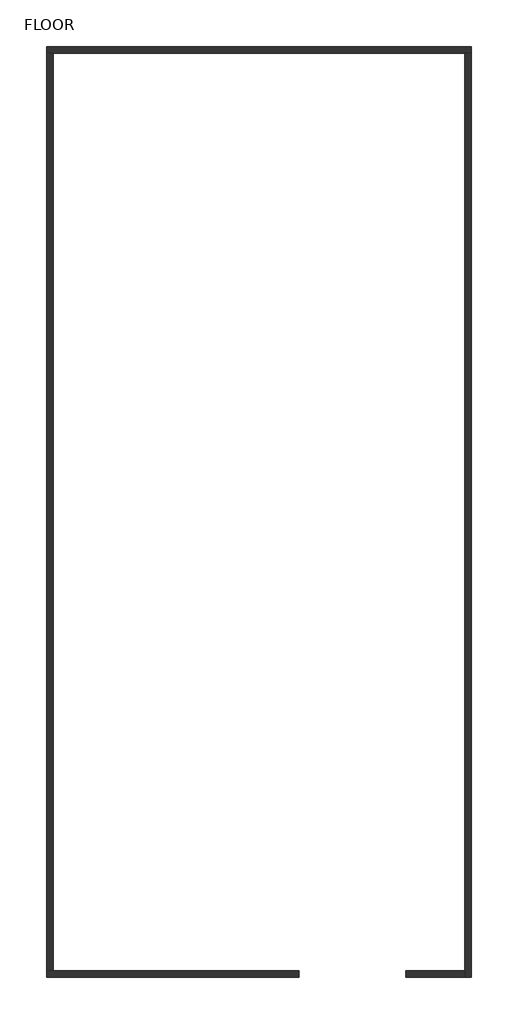
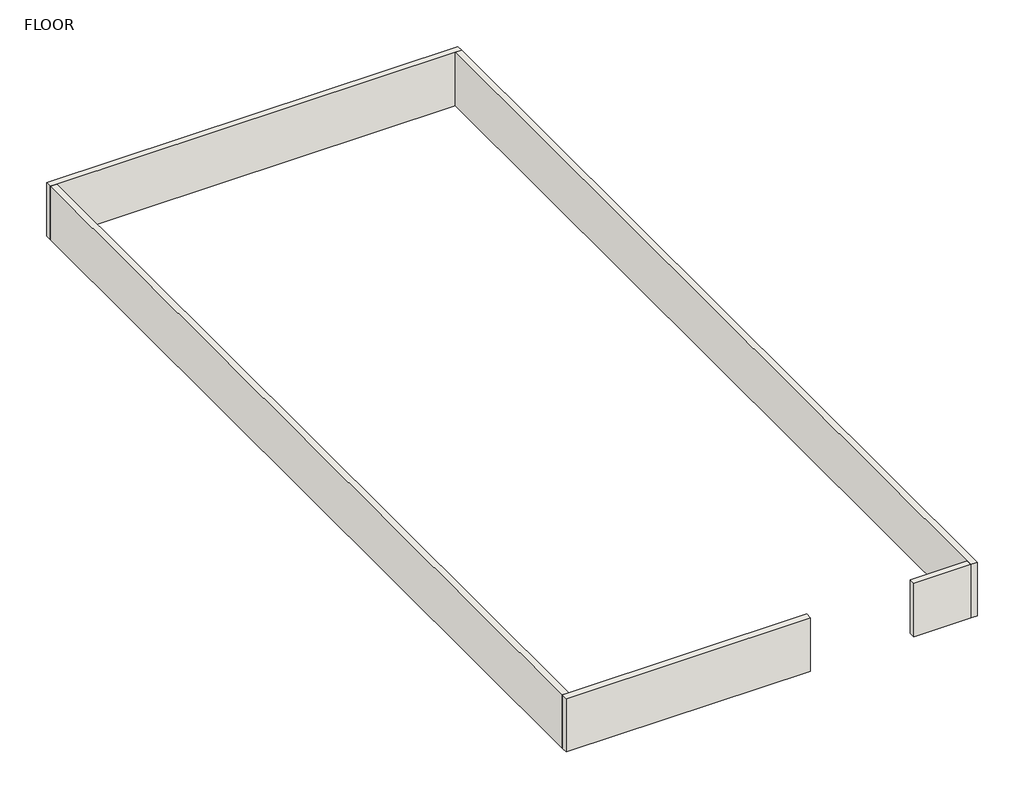
# One storey: 5 walls.
"""IFC4 building model written with IfcOpenShell, lengths in millimetres."""

from ifc_helpers import new_model, si_unit, frame, origin, place, context, project, spatial, polyline, outline, extrude, faceted_brep, element, save

model = new_model("IFC4")

# Units and contexts
model_context = context("Model", 3, world=origin())
ifc_project = project(units=[si_unit("LENGTHUNIT", "METRE", prefix="MILLI")], contexts=[model_context])

# Site, building, storey
site = spatial("IfcSite", under=ifc_project)
building = spatial("IfcBuilding", under=site)
storey = spatial("IfcBuildingStorey", under=building, Name="FLOOR", Elevation=-152.4)

# Walls
placement = place(None, origin())
element("IfcWall", 1, ObjectType="Generic - 140mm Masonry", at=placement, inside=storey, context=model_context, shape_type="Brep", body=[
    faceted_brep([(-6353.4317552, 8894.2726811, -152.4), (-6213.4317552, 8894.2726811, -152.4), (2380.1682448, 8894.2726811, -152.4), (2520.1682448, 8894.2726811, -152.4), (2520.1682448, 8894.2726811, 1066.8), (2380.1682448, 8894.2726811, 1066.8), (-6213.4317552, 8894.2726811, 1066.8), (-6353.4317552, 8894.2726811, 1066.8), (-6353.4317552, 9034.2726811, -152.4), (-6353.4317552, 9034.2726811, 1066.8), (2520.1682448, 9034.2726811, 1066.8), (2520.1682448, 9034.2726811, -152.4)], [[[0, 1, 2, 3, 4, 5, 6, 7]], [[8, 9, 10, 11]], [[3, 2, 1, 0, 8, 11]], [[7, 6, 5, 4, 10, 9]], [[0, 7, 9, 8]], [[4, 3, 11, 10]]]),
])
element("IfcWall", 2, ObjectType="Generic - 140mm Masonry", at=placement, inside=storey, context=model_context, shape_type="SweptSolid", body=[
    extrude(outline(polyline([(-6213.4317552, 8894.2726811), (-6213.4317552, -10249.3361723), (-6353.4317552, -10249.3361723), (-6353.4317552, 8894.2726811), (-6213.4317552, 8894.2726811)])), frame((0.0, 0.0, -152.4), z_axis=(0.0, 0.0, 1.0), x_axis=(1.0, 0.0, 0.0)), (0.0, 0.0, 1.0), 1219.2),
])
element("IfcWall", 3, ObjectType="Generic - 140mm Masonry", at=placement, inside=storey, context=model_context, shape_type="Brep", body=[
    faceted_brep([(2380.1682448, 8894.2726811, -152.4), (2380.1682448, -10249.3361723, -152.4), (2380.1682448, -10389.3361723, -152.4), (2380.1682448, -10389.3361723, 1066.8), (2380.1682448, -10249.3361723, 1066.8), (2380.1682448, 8894.2726811, 1066.8), (2520.1682448, 8894.2726811, -152.4), (2520.1682448, 8894.2726811, 1066.8), (2520.1682448, -10389.3361723, 1066.8), (2520.1682448, -10389.3361723, -152.4)], [[[0, 1, 2, 3, 4, 5]], [[6, 7, 8, 9]], [[2, 1, 0, 6, 9]], [[5, 4, 3, 8, 7]], [[3, 2, 9, 8]], [[0, 5, 7, 6]]]),
])
element("IfcWall", 4, ObjectType="Generic - 140mm Masonry", at=placement, inside=storey, context=model_context, shape_type="SweptSolid", body=[
    extrude(outline(polyline([(1150.1682448, -10249.3361723), (2380.1682448, -10249.3361723), (2380.1682448, -10389.3361723), (1150.1682448, -10389.3361723), (1150.1682448, -10249.3361723)])), frame((0.0, 0.0, -152.4), z_axis=(0.0, 0.0, 1.0), x_axis=(1.0, 0.0, 0.0)), (0.0, 0.0, 1.0), 1219.2),
])
element("IfcWall", 5, ObjectType="Generic - 140mm Masonry", at=placement, inside=storey, context=model_context, shape_type="Brep", body=[
    faceted_brep([(-6353.4317552, -10249.3361723, 1066.8), (-6213.4317552, -10249.3361723, 1066.8), (-1083.4317552, -10249.3361723, 1066.8), (-1083.4317552, -10249.3361723, -152.4), (-6213.4317552, -10249.3361723, -152.4), (-6353.4317552, -10249.3361723, -152.4), (-6353.4317552, -10389.3361723, 1066.8), (-6353.4317552, -10389.3361723, -152.4), (-1083.4317552, -10389.3361723, -152.4), (-1083.4317552, -10389.3361723, 1066.8)], [[[0, 1, 2, 3, 4, 5]], [[6, 7, 8, 9]], [[2, 1, 0, 6, 9]], [[5, 4, 3, 8, 7]], [[3, 2, 9, 8]], [[0, 5, 7, 6]]]),
])

save(model, "model.ifc")

# Revit data of these elements
# Type "Generic - 140mm Masonry"
#   Layers, outside or top first: 140 mm "Concrete Masonry Units" (function 1)
# Elements 1, 2, 3, 4, 5 (IfcWall, "Generic - 140mm Masonry")
#   Top Offset = 0 mm
#   Base Offset = 0 mm
#   Unconnected Height = 1219.2 mm
#   wall height = 1219.2 mm
#   Phase Created = New Construction
#   Base Constraint = FLOOR
#   Materials on its faces: "Concrete Masonry Units"
# Materials
#   "Concrete Masonry Units": class "Masonry", colour RGB 181 181 181, transparency 0, Description = "Concrete masonry units", Cost = 0
